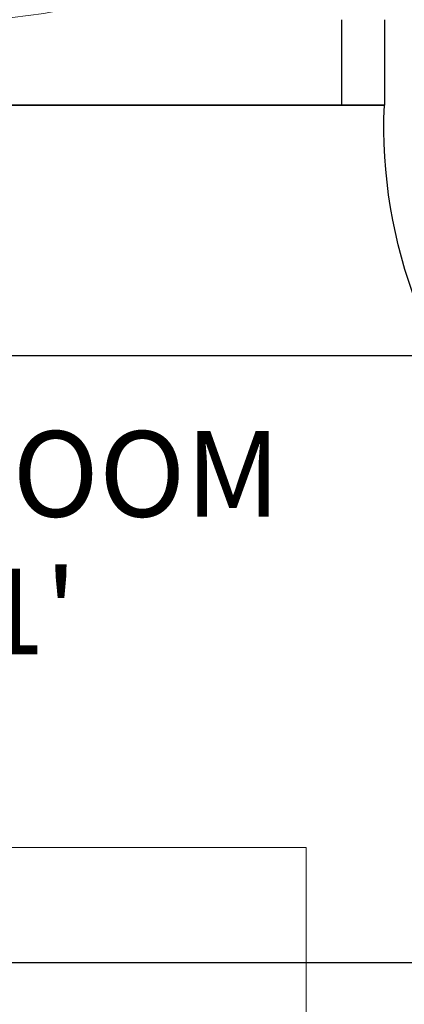
# Model space of a CAD drawing. Units: inches. Extents: x 4159 to 4826, y 299 to 1026.
# Tile 31 of 37: x 4590 to 4617, y 470 to 539. Entities that reach past the tile are written whole.
import ezdxf

# ---------------------------------------------------------------- set-up
doc = ezdxf.new("R2010")
doc.units = ezdxf.units.IN
for name, color, linetype, lineweight in [('A-ANNO-DIMS', 2, 'Continuous', 18), ('A-AREA-IDEN', 7, 'Continuous', 18), ('A-DOOR', 4, 'Continuous', 25), ('A-FURN', 8, 'Continuous', 18), ('A-WALL', 7, 'Continuous', 35)]:
    doc.layers.add(name, color=color, linetype=linetype, lineweight=lineweight)
doc.styles.get("Standard").update_dxf_attribs({"font": 'arial.ttf'})
doc.dimstyles.get("Standard").update_dxf_attribs({"dimtxt": 0.18, "dimasz": 0.18, "dimexe": 0.18, "dimexo": 0.0625, "dimgap": 0.09, "dimtad": 0, "dimtih": 1, "dimtoh": 1, "dimdec": 4, "dimzin": 0, "dimdsep": 46, "dimtxsty": 'Standard', "dimcen": 0.09, "dimadec": 0, "dimazin": 0, "dimtfac": 1, "dimtdec": 4, "dimtofl": 0, "dimtmove": 0, "dimatfit": 3, "dimfxl": 1, "dimtolj": 1, "dimtzin": 0, "dimarcsym": 0})

# ---------------------------------------------------------------- blocks, each defined once
blk = doc.blocks.new('Bed - Queen')
for p, q in [((0, -80.00003), (0, 0)), ((59.99999, -80.00003), (0, -80.00003))]:
    blk.add_line(p, q)
blk = doc.blocks.new('Sofa - Roundback Loveseat 5 ft.')
for p, q in [((0, -32.44198), (0, -5.99998)), ((-24, -33.99998), (-24, -11.46958)), ((24.00004, -33.99998), (24.00004, -11.46958)), ((-23.9998, -13.38178), (23.99986, -13.38178)), ((-24, -32.44198), (24.00004, -32.44198))]:
    blk.add_line(p, q)
for points in [[(-24, -33.99998), (-30, -33.99998), (-30, -7.99998)], [(30.00004, -7.99998), (30.00004, -33.99998), (24.00004, -33.99998)]]:
    blk.add_lwpolyline(points)
for centre, radius, start, end in [((0, -60.24998), 60.24998, 60.13715, 119.8628), ((0, -61.38438), 55.38444, 64.32083, 115.6792)]:
    blk.add_arc(centre, radius, start, end)
blk = doc.blocks.new('DOOR-SWING-36IN')
blk.add_lwpolyline([(0, 0), (-3, 0), (-3, 36), (0, 36)], close=True)
blk.add_arc((-1.5, 1.5), 34.533, 87.51045, 182.48955)
blk = doc.blocks.new('DOOR-FRAME-36IN')
for p, q in [((0, 6), (0, 0)), ((3, 6), (3, 0)), ((39, 6), (39, 0)), ((42, 6), (42, 0))]:
    blk.add_line(p, q)
blk = doc.blocks.new('*D54')
at = {"layer": 'A-ANNO-DIMS', "color": 0, "lineweight": -2, "transparency": 16777216}
for p, q in [((4501.373, 515.713), (4825.74, 515.713)), ((4825.56, 515.533), (4825.56, 494.636)), ((4825.56, 473.375), (4825.56, 494.272)), ((4541.952, 473.195), (4825.74, 473.195))]:
    blk.add_line(p, q, dxfattribs=at)
at = {"layer": 'A-ANNO-DIMS', "color": 0, "transparency": 16777216}
for points in [[(4825.53, 515.533), (4825.59, 515.533), (4825.56, 515.713)], [(4825.53, 473.375), (4825.59, 473.375), (4825.56, 473.195)]]:
    blk.add_solid(points, dxfattribs=at)
at = {"layer": 'Defpoints', "color": 0, "transparency": 16777216}
for p in [(4501.31, 515.713), (4825.56, 515.713), (4541.889, 473.195)]:
    blk.add_point(p, dxfattribs=at)
at = {"layer": 'A-ANNO-DIMS', "color": 0, "transparency": 16777216, "insert": (4825.56, 494.454), "char_height": 0.18, "attachment_point": 5}
blk.add_mtext('\\A1;42.52', dxfattribs=at)

msp = doc.modelspace()

# ---------------------------------------------------------------- linework, layer by layer
at = {"layer": 'A-WALL'}
msp.add_line((4615.31, 533.254), (4547.889, 533.254), dxfattribs=at)
msp.add_line((4615.31, 533.254), (4547.889, 533.254), dxfattribs=at)

# ---------------------------------------------------------------- block references
at = {"layer": 'A-DOOR'}
msp.add_blockref('DOOR-FRAME-36IN', (4612.31, 533.254), dxfattribs=at)
at = {"layer": 'A-DOOR', "extrusion": (0, 0, -1), "zscale": -1, "rotation": 180}
msp.add_blockref('DOOR-SWING-36IN', (-4651.31, 533.254), dxfattribs=at)
at = {"layer": 'A-FURN', "xscale": 0.5700533147329089, "yscale": 0.5700533147329089, "zscale": 0.5700533147329089, "rotation": 180}
msp.add_blockref('Sofa - Roundback Loveseat 5 ft.', (4585.903, 539.254), dxfattribs=at)
at = {"layer": 'A-FURN', "rotation": 180}
msp.add_blockref('Bed - Queen', (4609.814, 401.246), dxfattribs=at)

# ---------------------------------------------------------------- texts
at = {"layer": 'A-AREA-IDEN'}
for s, p in [('BED ROOM', (4566.36, 504.422)), ("10'X11'", (4566.36, 494.784))]:
    msp.add_text(s, height=6, dxfattribs=at).set_placement(p)

# ---------------------------------------------------------------- dimensions: what is measured, and where the dimension line sits
at = {"layer": 'A-ANNO-DIMS'}
dim = msp.add_linear_dim(base=(4825.56, 515.713), p1=(4541.889, 473.195), p2=(4501.31, 515.713), angle=90, dimstyle='Standard', override={"dimdec": 2, "dimlfac": 1, "dimrnd": 0, "dimzin": 0, "dimdsep": 46, "dimlunit": 2}, dxfattribs=at)
dim.commit()
dim.dimension.update_dxf_attribs({"geometry": '*D54', "text_midpoint": (4825.56, 494.454)})

doc.saveas('drawing.dxf')
